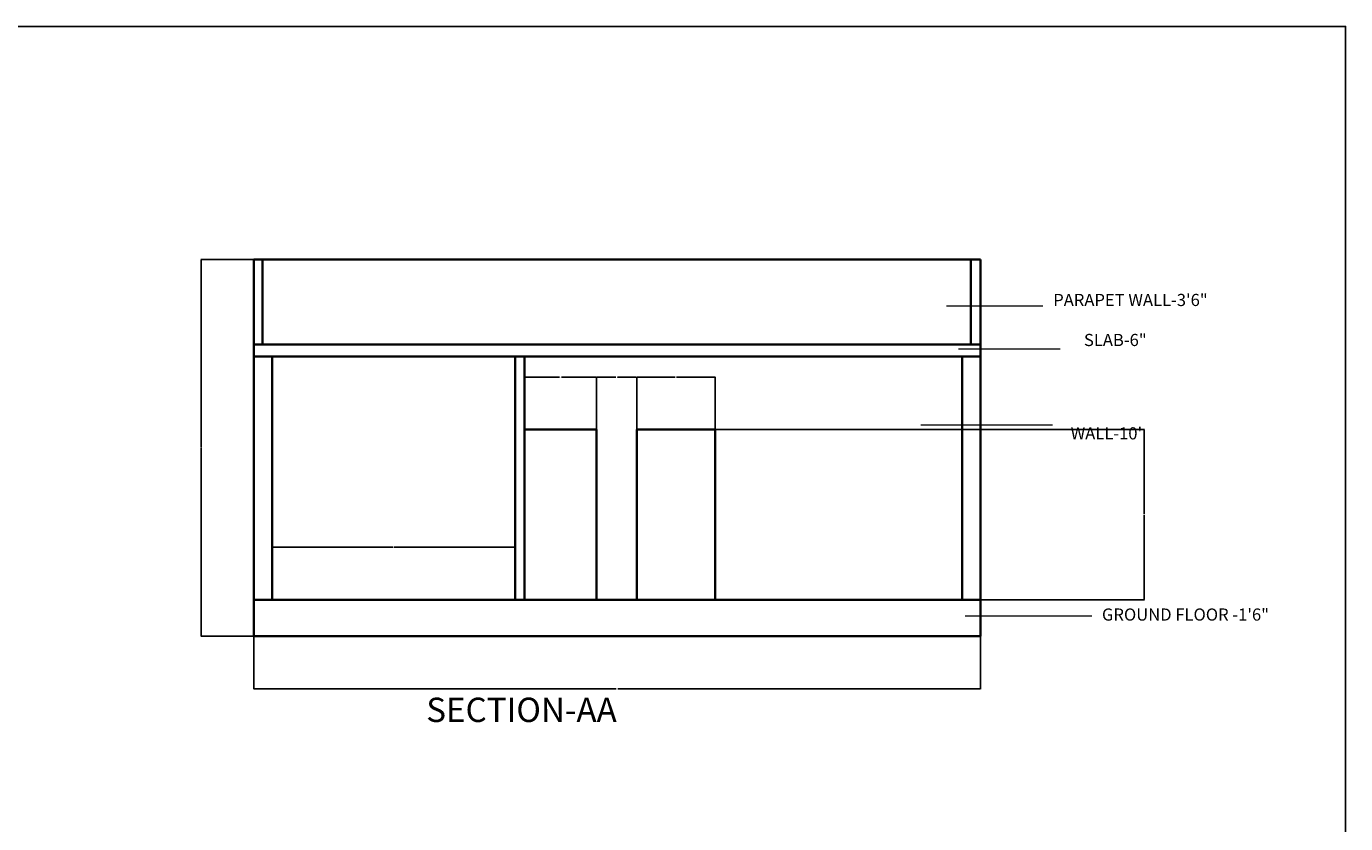
# Model space of a CAD drawing. Units: inches. Extents: x 1587 to 2880, y 1287 to 2423.
# Tile 8 of 8: x 2229 to 2880, y 2030 to 2423. Entities that reach past the tile are written whole.
import ezdxf

# ---------------------------------------------------------------- set-up
doc = ezdxf.new("R2010")
doc.units = ezdxf.units.IN
for name, color, linetype, lineweight in [('A-ANNO-DIMS', 2, 'Continuous', 18), ('A-ANNO-TEXT', 7, 'Continuous', 18), ('A-ANNO-TTLB', 7, 'Continuous', 25), ('A-SECT', 7, 'Continuous', 35)]:
    doc.layers.add(name, color=color, linetype=linetype, lineweight=lineweight)
doc.layers.add('A-WALL-PATT', color=251, linetype='Continuous', lineweight=13, true_color=0x636466)
doc.styles.get("Standard").update_dxf_attribs({"font": 'arial.ttf'})
doc.dimstyles.get("Standard").update_dxf_attribs({"dimtxt": 0.18, "dimasz": 0.18, "dimexe": 0.18, "dimexo": 0.0625, "dimgap": 0.09, "dimtad": 0, "dimtih": 1, "dimtoh": 1, "dimdec": 4, "dimzin": 0, "dimdsep": 46, "dimtxsty": 'Standard', "dimcen": 0.09, "dimadec": 0, "dimazin": 0, "dimtfac": 1, "dimtdec": 4, "dimtofl": 0, "dimtmove": 0, "dimatfit": 3, "dimfxl": 1, "dimtolj": 1, "dimtzin": 0, "dimarcsym": 0})

# ---------------------------------------------------------------- blocks, each defined once
blk = doc.blocks.new('*D93')
at = {"layer": 'A-ANNO-DIMS', "color": 0, "lineweight": -2, "transparency": 16777216}
for p, q in [((2341.53, 2122.09), (2341.53, 2096.07)), ((2700.03, 2122.09), (2700.03, 2096.07)), ((2341.71, 2096.25), (2520.39, 2096.25)), ((2699.85, 2096.25), (2521.18, 2096.25))]:
    blk.add_line(p, q, dxfattribs=at)
at = {"layer": 'A-ANNO-DIMS', "color": 0, "transparency": 16777216}
for points in [[(2341.71, 2096.28), (2341.71, 2096.22), (2341.53, 2096.25)], [(2699.85, 2096.28), (2699.85, 2096.22), (2700.03, 2096.25)]]:
    blk.add_solid(points, dxfattribs=at)
at = {"layer": 'Defpoints', "color": 0, "transparency": 16777216}
for p in [(2341.53, 2122.15), (2700.03, 2122.15), (2700.03, 2096.25)]:
    blk.add_point(p, dxfattribs=at)
at = {"layer": 'A-ANNO-DIMS', "color": 0, "transparency": 16777216, "insert": (2520.78, 2096.25), "char_height": 0.18, "attachment_point": 5}
blk.add_mtext('\\A1;358.5', dxfattribs=at)
blk = doc.blocks.new('*D94')
at = {"layer": 'A-ANNO-DIMS', "color": 0, "lineweight": -2, "transparency": 16777216}
for p, q in [((2341.47, 2308.15), (2315.45, 2308.15)), ((2315.63, 2307.97), (2315.63, 2215.33)), ((2315.63, 2122.33), (2315.63, 2214.97)), ((2341.47, 2122.15), (2315.45, 2122.15))]:
    blk.add_line(p, q, dxfattribs=at)
at = {"layer": 'A-ANNO-DIMS', "color": 0, "transparency": 16777216}
for points in [[(2315.6, 2307.97), (2315.66, 2307.97), (2315.63, 2308.15)], [(2315.6, 2122.33), (2315.66, 2122.33), (2315.63, 2122.15)]]:
    blk.add_solid(points, dxfattribs=at)
at = {"layer": 'Defpoints', "color": 0, "transparency": 16777216}
for p in [(2315.63, 2308.15), (2341.53, 2308.15), (2341.53, 2122.15)]:
    blk.add_point(p, dxfattribs=at)
at = {"layer": 'A-ANNO-DIMS', "color": 0, "transparency": 16777216, "insert": (2315.63, 2215.15), "char_height": 0.18, "attachment_point": 5}
blk.add_mtext('\\A1;186', dxfattribs=at)
blk = doc.blocks.new('*D95')
at = {"layer": 'A-ANNO-DIMS', "color": 0, "lineweight": -2, "transparency": 16777216}
for p, q in [((2350.53, 2140.21), (2350.53, 2166.23)), ((2350.71, 2166.05), (2410.25, 2166.05)), ((2470.35, 2166.05), (2410.81, 2166.05)), ((2470.53, 2140.21), (2470.53, 2166.23))]:
    blk.add_line(p, q, dxfattribs=at)
at = {"layer": 'A-ANNO-DIMS', "color": 0, "transparency": 16777216}
for points in [[(2350.71, 2166.08), (2350.71, 2166.02), (2350.53, 2166.05)], [(2470.35, 2166.08), (2470.35, 2166.02), (2470.53, 2166.05)]]:
    blk.add_solid(points, dxfattribs=at)
at = {"layer": 'Defpoints', "color": 0, "transparency": 16777216}
for p in [(2470.53, 2166.05), (2350.53, 2140.15), (2470.53, 2140.15)]:
    blk.add_point(p, dxfattribs=at)
at = {"layer": 'A-ANNO-DIMS', "color": 0, "transparency": 16777216, "insert": (2410.53, 2166.05), "char_height": 0.18, "attachment_point": 5}
blk.add_mtext('\\A1;120', dxfattribs=at)
blk = doc.blocks.new('*D96')
at = {"layer": 'A-ANNO-DIMS', "color": 0, "lineweight": -2, "transparency": 16777216}
for p, q in [((2475.03, 2224.21), (2475.03, 2250.23)), ((2475.21, 2250.05), (2492.36, 2250.05)), ((2510.43, 2250.05), (2493.29, 2250.05)), ((2510.61, 2224.21), (2510.61, 2250.23))]:
    blk.add_line(p, q, dxfattribs=at)
at = {"layer": 'A-ANNO-DIMS', "color": 0, "transparency": 16777216}
for points in [[(2475.21, 2250.08), (2475.21, 2250.02), (2475.03, 2250.05)], [(2510.43, 2250.08), (2510.43, 2250.02), (2510.61, 2250.05)]]:
    blk.add_solid(points, dxfattribs=at)
at = {"layer": 'Defpoints', "color": 0, "transparency": 16777216}
for p in [(2510.61, 2250.05), (2475.03, 2224.15), (2510.61, 2224.15)]:
    blk.add_point(p, dxfattribs=at)
at = {"layer": 'A-ANNO-DIMS', "color": 0, "transparency": 16777216, "insert": (2492.82, 2250.05), "char_height": 0.18, "attachment_point": 5}
blk.add_mtext('\\A1;35.575', dxfattribs=at)
blk = doc.blocks.new('*D97')
at = {"layer": 'A-ANNO-DIMS', "color": 0, "lineweight": -2, "transparency": 16777216}
for p, q in [((2510.61, 2224.21), (2510.61, 2250.23)), ((2510.79, 2250.05), (2520.14, 2250.05)), ((2530.27, 2250.05), (2520.91, 2250.05)), ((2530.45, 2224.21), (2530.45, 2250.23))]:
    blk.add_line(p, q, dxfattribs=at)
at = {"layer": 'A-ANNO-DIMS', "color": 0, "transparency": 16777216}
for points in [[(2510.79, 2250.08), (2510.79, 2250.02), (2510.61, 2250.05)], [(2530.27, 2250.08), (2530.27, 2250.02), (2530.45, 2250.05)]]:
    blk.add_solid(points, dxfattribs=at)
at = {"layer": 'Defpoints', "color": 0, "transparency": 16777216}
for p in [(2530.45, 2250.05), (2510.61, 2224.15), (2530.45, 2224.15)]:
    blk.add_point(p, dxfattribs=at)
at = {"layer": 'A-ANNO-DIMS', "color": 0, "transparency": 16777216, "insert": (2520.53, 2250.05), "char_height": 0.18, "attachment_point": 5}
blk.add_mtext('\\A1;19.84', dxfattribs=at)
blk = doc.blocks.new('*D98')
at = {"layer": 'A-ANNO-DIMS', "color": 0, "lineweight": -2, "transparency": 16777216}
for p, q in [((2569.21, 2224.15), (2781, 2224.15)), ((2780.82, 2223.97), (2780.82, 2182.33)), ((2780.82, 2140.33), (2780.82, 2181.97)), ((2569.21, 2140.15), (2781, 2140.15))]:
    blk.add_line(p, q, dxfattribs=at)
at = {"layer": 'A-ANNO-DIMS', "color": 0, "transparency": 16777216}
for points in [[(2780.79, 2223.97), (2780.85, 2223.97), (2780.82, 2224.15)], [(2780.79, 2140.33), (2780.85, 2140.33), (2780.82, 2140.15)]]:
    blk.add_solid(points, dxfattribs=at)
at = {"layer": 'Defpoints', "color": 0, "transparency": 16777216}
for p in [(2569.14, 2224.15), (2780.82, 2224.15), (2569.14, 2140.15)]:
    blk.add_point(p, dxfattribs=at)
at = {"layer": 'A-ANNO-DIMS', "color": 0, "transparency": 16777216, "insert": (2780.82, 2182.15), "char_height": 0.18, "attachment_point": 5}
blk.add_mtext('\\A1;84', dxfattribs=at)
blk = doc.blocks.new('*D99')
at = {"layer": 'A-ANNO-DIMS', "color": 0, "lineweight": -2, "transparency": 16777216}
for p, q in [((2530.45, 2224.21), (2530.45, 2250.23)), ((2530.63, 2250.05), (2549.47, 2250.05)), ((2568.96, 2250.05), (2550.12, 2250.05)), ((2569.14, 2224.21), (2569.14, 2250.23))]:
    blk.add_line(p, q, dxfattribs=at)
at = {"layer": 'A-ANNO-DIMS', "color": 0, "transparency": 16777216}
for points in [[(2530.63, 2250.08), (2530.63, 2250.02), (2530.45, 2250.05)], [(2568.96, 2250.08), (2568.96, 2250.02), (2569.14, 2250.05)]]:
    blk.add_solid(points, dxfattribs=at)
at = {"layer": 'Defpoints', "color": 0, "transparency": 16777216}
for p in [(2569.14, 2250.05), (2530.45, 2224.15), (2569.14, 2224.15)]:
    blk.add_point(p, dxfattribs=at)
at = {"layer": 'A-ANNO-DIMS', "color": 0, "transparency": 16777216, "insert": (2549.8, 2250.05), "char_height": 0.18, "attachment_point": 5}
blk.add_mtext('\\A1;38.7', dxfattribs=at)

msp = doc.modelspace()

# ---------------------------------------------------------------- hatches: boundary and pattern name
at = {"layer": 'A-WALL-PATT'}
h = msp.add_hatch(color=256, dxfattribs=at)
h.dxf.hatch_style = 1
h.paths.add_polyline_path([(2190.3423, 1988.3868), (2181.3423, 1988.3868), (2137.8423, 1988.3868), (1779.3423, 1988.3868), (1779.3423, 1939.6287), (1788.3423, 1939.6287), (1788.3423, 1979.3868), (1956.3423, 1979.3868), (1956.3423, 1841.3868), (1948.4175, 1841.3868), (1948.4175, 1836.8868), (1968.256, 1836.8868), (1968.256, 1839.1368), (1968.256, 1841.3868), (1960.8423, 1841.3868), (1960.8423, 1979.3868), (2128.8423, 1979.3868), (2128.8423, 1971.4394), (2133.3423, 1971.4394), (2133.3423, 1979.3868), (2181.3423, 1979.3868), (2181.3423, 1895.3868), (2174.9842, 1895.3868), (2174.9842, 1886.3868), (2190.3423, 1886.3868), (2190.3423, 1895.3868)])
h.paths.add_polyline_path([(1788.3423, 1879.6287), (1779.3423, 1879.6287), (1779.3423, 1827.4437), (1788.3423, 1827.4437), (1788.3423, 1836.8868), (1839.8915, 1836.8868), (1839.8915, 1839.1368), (1839.8915, 1841.3868), (1788.3423, 1841.3868)])
h.paths.add_polyline_path([(1876.8423, 1836.8868), (1908.901, 1836.8868), (1908.901, 1839.1368), (1908.901, 1841.3868), (1866.9993, 1841.3868), (1866.9993, 1836.8868), (1872.3423, 1836.8868), (1872.3423, 1776.8868), (1788.3423, 1776.8868), (1788.3423, 1803.4437), (1779.3423, 1803.4437), (1779.3423, 1757.1447), (1788.3423, 1757.1447), (1788.3423, 1772.3868), (1872.3423, 1772.3868), (1872.3423, 1712.3868), (1867.9542, 1712.3868), (1867.9542, 1707.8868), (1876.8423, 1707.8868), (1876.8423, 1772.3868)])
h.paths.add_polyline_path([(1842.6206, 1710.1368), (1842.6206, 1712.3868), (1788.3423, 1712.3868), (1788.3423, 1733.1447), (1779.3423, 1733.1447), (1779.3423, 1678.6557), (1788.3423, 1678.6557), (1788.3423, 1707.8868), (1842.6206, 1707.8868)])
h.paths.add_polyline_path([(1912.8423, 1712.3868), (1908.3423, 1712.3868), (1876.8423, 1712.3868), (1876.8423, 1707.8868), (1908.3423, 1707.8868), (1908.3423, 1702.2679), (1912.8423, 1702.2679)])
h.paths.add_polyline_path([(2137.8423, 1844.5168), (2128.8423, 1844.5168), (2128.8423, 1841.3868), (2006.9533, 1841.3868), (2006.9533, 1836.8868), (2128.8423, 1836.8868), (2128.8423, 1832.632), (2137.8423, 1832.632)])
h.paths.add_polyline_path([(1997.6598, 1534.8868), (1997.6598, 1539.3868), (1912.8423, 1539.3868), (1912.8423, 1543.4794), (1903.8423, 1543.4794), (1903.8423, 1530.3868), (1997.6598, 1530.3868)])
h.paths.add_polyline_path([(1912.8423, 1666.7101), (1910.5923, 1666.7101), (1908.3423, 1666.7101), (1908.3423, 1587.8868), (1903.8423, 1587.8868), (1879.6624, 1587.8868), (1879.6624, 1578.8868), (1903.8423, 1578.8868), (1903.8423, 1574.5584), (1912.8423, 1574.5584), (1912.8423, 1578.8868), (1912.8423, 1587.8868)])
h.paths.add_polyline_path([(1788.3423, 1618.6557), (1779.3423, 1618.6557), (1779.3423, 1578.8868), (1819.6624, 1578.8868), (1819.6624, 1583.3868), (1819.6624, 1587.8868), (1788.3423, 1587.8868)])
h.paths.add_polyline_path([(2133.3423, 1945.4046), (2131.0923, 1945.4046), (2128.8423, 1945.4046), (2128.8423, 1880.5168), (2137.8423, 1880.5168), (2137.8423, 1886.3868), (2150.9842, 1886.3868), (2150.9842, 1890.8868), (2150.9842, 1895.3868), (2133.3423, 1895.3868)], flags=17)
h.paths.add_polyline_path([(2137.8423, 1788.9874), (2133.3423, 1788.9874), (2128.8423, 1788.9874), (2128.8423, 1699.8868), (2006.9533, 1699.8868), (2006.9533, 1695.3868), (2128.8423, 1695.3868), (2128.8423, 1539.3868), (2057.6598, 1539.3868), (2057.6598, 1530.3868), (2128.8423, 1530.3868), (2128.8423, 1461.3868), (1988.2941, 1461.3868), (1988.2941, 1452.3868), (2137.8423, 1452.3868), (2137.8423, 1530.3868)])
h.paths.add_polyline_path([(1866.9166, 1348.94), (2042.3313, 1348.94), (2042.3313, 1371.6078), (1866.9166, 1371.6078)], flags=9)
h.paths.add_polyline_path([(2758.0473, 2126.4845), (2848.522, 2126.4845), (2848.522, 2138.8487), (2758.0473, 2138.8487)], flags=9)
h.paths.add_polyline_path([(2742.9428, 2216.0014), (2782.483, 2216.0014), (2782.483, 2228.3657), (2742.9428, 2228.3657)], flags=9)
h.paths.add_polyline_path([(2749.234, 2261.9992), (2784.0963, 2261.9992), (2784.0963, 2274.3634), (2749.234, 2274.3634)], flags=9)
h.paths.add_polyline_path([(2733.8012, 2281.8262), (2817.7726, 2281.8262), (2817.7726, 2294.1904), (2733.8012, 2294.1904)], flags=9)
h.paths.add_polyline_path([(2422.857, 2073.081), (2531.34, 2073.081), (2531.34, 2097.8095), (2422.857, 2097.8095)], flags=9)
h.paths.add_polyline_path([(1856.7732, 2082.3109), (1956.866, 2082.3109), (1956.866, 2107.0394), (1856.7732, 2107.0394)], flags=9)
h.paths.add_polyline_path([(2777.4581, 1646.9437), (2794.6887, 1646.9437), (2794.6887, 1671.6723), (2777.4581, 1671.6723)], flags=9)
h.paths.add_polyline_path([(2585.5416, 1728.5169), (2655.2006, 1728.5169), (2655.2006, 1760.9057), (2585.5416, 1760.9057)], flags=9)
h.paths.add_polyline_path([(2554.1301, 1617.6432), (2608.2079, 1617.6432), (2608.2079, 1640.032), (2554.1301, 1640.032)], flags=9)
h.paths.add_polyline_path([(2359.8658, 1678.1191), (2437.8454, 1678.1191), (2437.8454, 1700.5079), (2359.8658, 1700.5079)], flags=9)
h.paths.add_polyline_path([(2392.0171, 1749.26), (2422.3411, 1749.26), (2422.3411, 1767.9173), (2392.0171, 1767.9173)], flags=9)
h.paths.add_polyline_path([(2391.9937, 1787.5799), (2422.3177, 1787.5799), (2422.3177, 1806.2373), (2391.9937, 1806.2373)], flags=9)
h.paths.add_polyline_path([(2707.7632, 1927.6903), (2738.1623, 1927.6903), (2738.1623, 1946.3477), (2707.7632, 1946.3477)], flags=9)
h.paths.add_polyline_path([(2581.5534, 1846.9887), (2635.6148, 1846.9887), (2635.6148, 1869.3775), (2581.5534, 1869.3775)], flags=9)
h.paths.add_polyline_path([(2382.3802, 1864.4978), (2436.4416, 1864.4978), (2436.4416, 1886.8866), (2382.3802, 1886.8866)], flags=9)
h.paths.add_polyline_path([(2023.35, 1728.5169), (2093.0089, 1728.5169), (2093.0089, 1760.9057), (2023.35, 1760.9057)], flags=25)
h.paths.add_polyline_path([(1991.9385, 1617.6432), (2046.0162, 1617.6432), (2046.0162, 1640.032), (1991.9385, 1640.032)], flags=25)
h.paths.add_polyline_path([(1791.1103, 1678.1191), (1869.0899, 1678.1191), (1869.0899, 1700.5079), (1791.1103, 1700.5079)], flags=9)
h.paths.add_polyline_path([(1829.8255, 1749.26), (1860.1495, 1749.26), (1860.1495, 1767.9173), (1829.8255, 1767.9173)], flags=25)
h.paths.add_polyline_path([(1829.8021, 1787.5799), (1860.1261, 1787.5799), (1860.1261, 1806.2373), (1829.8021, 1806.2373)], flags=25)
h.paths.add_polyline_path([(2145.5716, 1927.6903), (2175.9706, 1927.6903), (2175.9706, 1946.3477), (2145.5716, 1946.3477)], flags=25)
h.paths.add_polyline_path([(2019.3617, 1846.9887), (2073.4231, 1846.9887), (2073.4231, 1869.3775), (2019.3617, 1869.3775)], flags=25)
h.paths.add_polyline_path([(1820.1886, 1864.4978), (1874.25, 1864.4978), (1874.25, 1886.8866), (1820.1886, 1886.8866)], flags=25)

# ---------------------------------------------------------------- linework, layer by layer
at = {"layer": 'A-ANNO-TEXT'}
for p, q in [((2683.2593, 2285.2191), (2730.8859, 2285.2191)), ((2689.2524, 2264.0791), (2739.3173, 2264.0791)), ((2670.6788, 2226.5055), (2735.5919, 2226.5055)), ((2692.4454, 2132.2352), (2754.9234, 2132.2352))]:
    msp.add_line(p, q, dxfattribs=at)
at = {"layer": 'A-ANNO-TTLB'}
msp.add_lwpolyline([(1586.5185, 2423.1539), (2880.2062, 2423.1539), (2880.2062, 1286.9347), (1586.5185, 1286.9347)], close=True, dxfattribs=at)
at = {"layer": 'A-SECT'}
for p, q in [((2341.534, 2308.1515), (2341.534, 2122.1515)), ((2341.534, 2308.1515), (2700.034, 2308.1515)), ((2345.9146, 2266.1515), (2345.9146, 2308.1515)), ((2695.2302, 2266.1515), (2695.2302, 2308.1515)), ((2700.034, 2308.1515), (2700.034, 2122.1515)), ((2341.534, 2266.1515), (2700.034, 2266.1515)), ((2341.534, 2260.1515), (2700.034, 2260.1515)), ((2350.534, 2260.1515), (2350.534, 2140.1515)), ((2470.534, 2260.1515), (2470.534, 2140.1515)), ((2475.034, 2260.1515), (2475.034, 2140.1515)), ((2691.034, 2260.1515), (2691.034, 2140.1515)), ((2475.034, 2224.1515), (2510.6092, 2224.1515)), ((2510.6092, 2224.1515), (2510.6092, 2140.1515)), ((2530.4477, 2224.1515), (2530.4477, 2140.1515)), ((2530.4477, 2224.1515), (2569.145, 2224.1515)), ((2569.145, 2224.1515), (2569.145, 2140.1515)), ((2341.534, 2140.1515), (2700.034, 2140.1515)), ((2341.534, 2122.1515), (2700.034, 2122.1515))]:
    msp.add_line(p, q, dxfattribs=at)

# ---------------------------------------------------------------- texts
at = {"layer": 'A-ANNO-TEXT', "attachment_point": 1}
for s, width, insert, char_height in [('PARAPET WALL-3\'6"', 117.931683, (2735.9479, 2291.127), 6), ('SLAB-6"', 57.740547, (2751.1106, 2271.3778), 6), ("WALL-10'", 66.539917, (2744.5451, 2225.3022), 6), ('GROUND FLOOR -1\'6"', 92.515548, (2759.9934, 2135.8671), 6), ('SECTION-AA', 209.309093, (2426.6101, 2091.8464), 12)]:
    msp.add_mtext_dynamic_manual_height_columns(s, width=width, gutter_width=12.5, heights=[0], dxfattribs=dict(at, insert=insert, char_height=char_height))

# ---------------------------------------------------------------- dimensions: what is measured, and where the dimension line sits
at = {"layer": 'A-ANNO-DIMS'}
for base, p1, p2, angle, override, picture, middle in [((2315.634, 2308.1515), (2341.534, 2122.1515), (2341.534, 2308.1515), 90, {"dimdec": 0, "dimlfac": 1, "dimrnd": 0, "dimzin": 0, "dimdsep": 46, "dimlunit": 2}, '*D94', (2315.634, 2215.1515)), ((2530.4477, 2250.0515), (2510.6092, 2224.1515), (2530.4477, 2224.1515), 0, {"dimdec": 2, "dimlfac": 1, "dimrnd": 0, "dimzin": 0, "dimdsep": 46, "dimlunit": 2}, '*D97', (2520.5285, 2250.0515)), ((2780.8234, 2224.1515), (2569.145, 2140.1515), (2569.145, 2224.1515), 90, {"dimdec": 0, "dimlfac": 1, "dimrnd": 0, "dimzin": 0, "dimdsep": 46, "dimlunit": 2}, '*D98', (2780.8234, 2182.1515))]:
    dim = msp.add_linear_dim(base=base, p1=p1, p2=p2, angle=angle, dimstyle='Standard', override=override, dxfattribs=at)
    dim.commit()
    dim.dimension.update_dxf_attribs({"geometry": picture, "text_midpoint": middle})
for base, p1, p2, override, picture, middle in [((2510.6092, 2250.0515), (2475.034, 2224.1515), (2510.6092, 2224.1515), {"dimdec": 3, "dimlfac": 1, "dimrnd": 0, "dimzin": 0, "dimdsep": 46, "dimlunit": 2}, '*D96', (2492.8216, 2250.0515)), ((2569.145, 2250.0515), (2530.4477, 2224.1515), (2569.145, 2224.1515), {"dimdec": 1, "dimlfac": 1, "dimrnd": 0, "dimzin": 0, "dimdsep": 46, "dimlunit": 2}, '*D99', (2549.7963, 2250.0515)), ((2470.534, 2166.0515), (2350.534, 2140.1515), (2470.534, 2140.1515), {"dimdec": 0, "dimlfac": 1, "dimrnd": 0, "dimzin": 0, "dimdsep": 46, "dimlunit": 2}, '*D95', (2410.534, 2166.0515)), ((2700.034, 2096.2515), (2341.534, 2122.1515), (2700.034, 2122.1515), {"dimdec": 1, "dimlfac": 1, "dimrnd": 0, "dimzin": 0, "dimdsep": 46, "dimlunit": 2}, '*D93', (2520.784, 2096.2515))]:
    dim = msp.add_linear_dim(base=base, p1=p1, p2=p2, dimstyle='Standard', override=override, dxfattribs=at)
    dim.commit()
    dim.dimension.update_dxf_attribs({"geometry": picture, "text_midpoint": middle})

doc.saveas('drawing.dxf')
